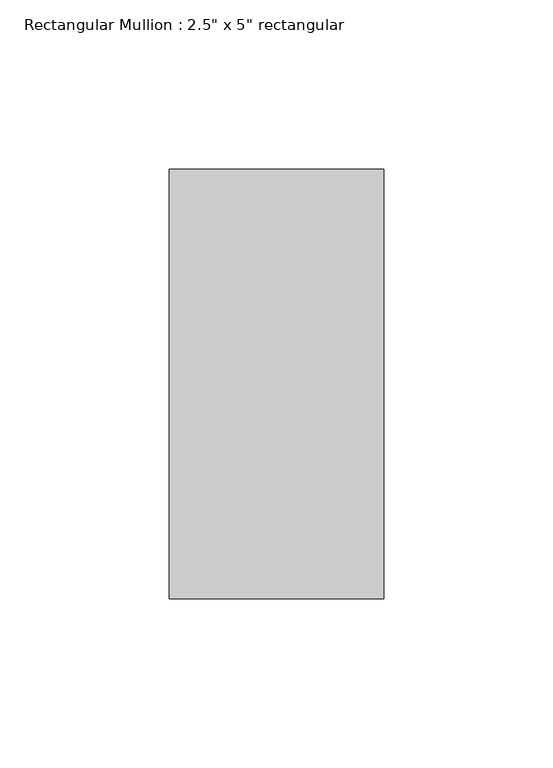
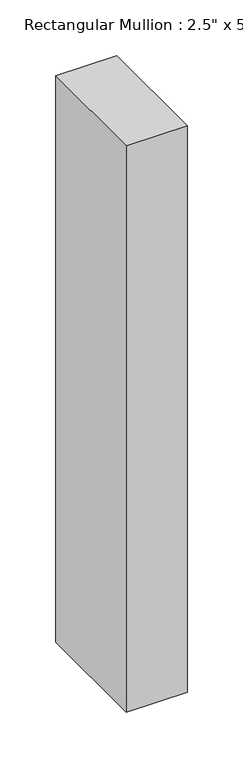
"""IFC4 building model written with IfcOpenShell, lengths in millimetres: member geometry."""

from ifc_helpers import new_model, si_unit, frame, origin, place, context, project, spatial, polyline, outline, extrude, source, transform, mapped, element, save


def member_081e0693(model_context):
    return source(origin(), model_context, "Body", "SweptSolid", [
        extrude(outline(polyline([(0.0, 63.5), (0.0, -63.5), (-63.5, -63.5), (-63.5, 63.5), (0.0, 63.5)])), frame((0.0, 0.0, -622.3), z_axis=(0.0, 0.0, 1.0), x_axis=(1.0, 0.0, 0.0)), (0.0, 0.0, 1.0), 622.3),
    ])


if __name__ == "__main__":
    model = new_model("IFC4")
    model_context = context("Model", 3, world=origin())
    ifc_project = project(units=[si_unit("LENGTHUNIT", "METRE", prefix="MILLI")], contexts=[model_context])
    site = spatial("IfcSite", under=ifc_project)
    building = spatial("IfcBuilding", under=site)
    placement = place(None, origin())
    member_shape = member_081e0693(model_context)
    element("IfcMember", 1, ObjectType="Rectangular Mullion : 2.5\" x 5\" rectangular", at=placement, inside=building, context=model_context, shape_type="MappedRepresentation", body=[
        mapped(member_shape, transform((0.0, 0.0, 0.0), x_axis=(1.0, 0.0, 0.0), y_axis=(0.0, 1.0, 0.0), z_axis=(0.0, 0.0, 1.0))),
    ])
    save(model, "model.ifc")

# Revit data of these elements
# Type "Rectangular Mullion : 2.5\" x 5\" rectangular"
#   built-in parameter 1007304 = 0.416667 (stored number, unit not read)
#   built-in parameter 1007301 = 0.104167 (stored number, unit not read)
#   built-in parameter 1007300 = 0.104167 (stored number, unit not read)
# Element 1 (IfcMember, "Rectangular Mullion : 2.5\" x 5\" rectangular")
#   Materials on its faces: "Aluminum"
# Materials
#   "Aluminum": class "Metal", colour RGB 247 247 247, transparency 0, Description = "Aluminum 6061", Cost = 0
